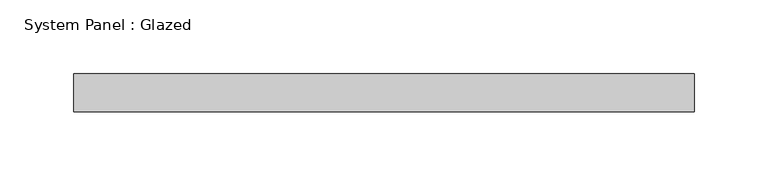
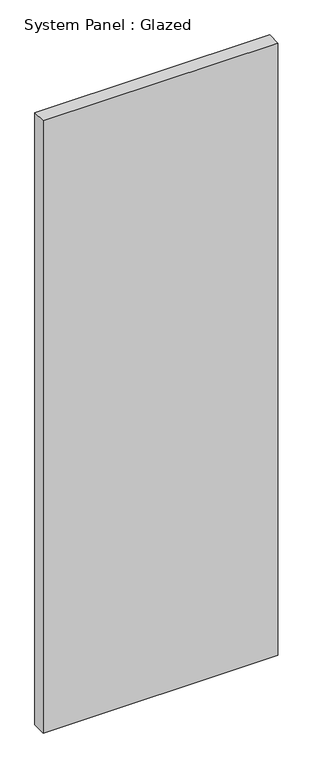
"""IFC4 building model written with IfcOpenShell, lengths in millimetres: plate geometry, System Panel : Glazed."""

from ifc_helpers import new_model, si_unit, origin, origin_with_axes, place, context, project, spatial, polyline, outline, extrude, source, transform, mapped, element, save


def system_panel_glazed_fe17e9eb(model_context):
    return source(origin(), model_context, "Body", "SweptSolid", [
        extrude(outline(polyline([(209.55, 19.05), (-209.55, 19.05), (-209.55, 44.45), (209.55, 44.45), (209.55, 19.05)])), origin_with_axes(), (0.0, 0.0, 1.0), 1155.7),
    ])


if __name__ == "__main__":
    model = new_model("IFC4")
    model_context = context("Model", 3, world=origin())
    ifc_project = project(units=[si_unit("LENGTHUNIT", "METRE", prefix="MILLI")], contexts=[model_context])
    site = spatial("IfcSite", under=ifc_project)
    building = spatial("IfcBuilding", under=site)
    placement = place(None, origin())
    system_panel_glazed_shape = system_panel_glazed_fe17e9eb(model_context)
    element("IfcPlate", 1, ObjectType="System Panel : Glazed", at=placement, inside=building, context=model_context, shape_type="MappedRepresentation", body=[
        mapped(system_panel_glazed_shape, transform((0.0, 0.0, 0.0), x_axis=(1.0, 0.0, 0.0), y_axis=(0.0, 1.0, 0.0), z_axis=(0.0, 0.0, 1.0))),
    ])
    save(model, "model.ifc")

# Revit data of these elements
# Type "System Panel : Glazed"
#   Construction Type Id = "GSP4R"
#   Analytic Construction = "1/8 in Pilkington single glazing"
#   Visual Light Transmittance = 0.9
#   Solar Heat Gain Coefficient = 0.86
#   Heat Transfer Coefficient (U) = 1.18115 BTU/(h·ft²·°F)
#   Define Thermal Properties by = 1
# Element 1 (IfcPlate, "System Panel : Glazed")
#   Materials on its faces: "Glass"
# Materials
#   "Glass": class "Glass", colour RGB 0 128 192, transparency 0.75, Description = "Soda Lime Glass", Cost = 0
